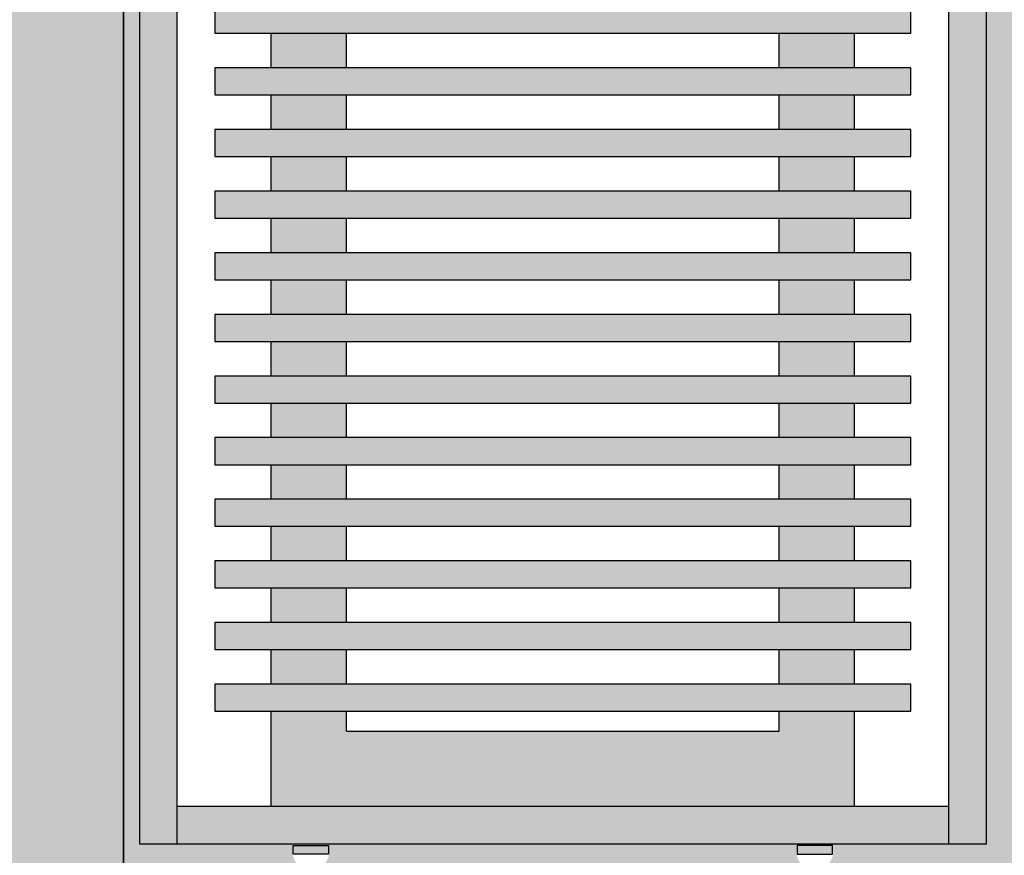
# Model space of a CAD drawing. Units: inches. Extents: x 1704 to 6393, y -157 to 1172.
# Tile 27 of 122: x 2351 to 2377, y 272 to 295. Entities that reach past the tile are written whole.
import ezdxf

# ---------------------------------------------------------------- set-up
doc = ezdxf.new("R2010")
doc.units = ezdxf.units.IN
doc.header["$MEASUREMENT"] = 0
for name, color, linetype, lineweight in [('A-ANNO-DIMS', 7, 'Continuous', 13), ('A-FURN', 8, 'Continuous', 18), ('A-WALL-PATT', 7, 'Continuous', 13), ('estofado', 7, 'Continuous', 25), ('WALLS', 7, 'Continuous', 35)]:
    doc.layers.add(name, color=color, linetype=linetype, lineweight=lineweight)
doc.layers.add('A-FLOR-PATT', color=7, linetype='Continuous', lineweight=13, true_color=0xf2f2f2)
doc.layers.add('MOBIL', color=7, linetype='Continuous')
doc.styles.get("Standard").update_dxf_attribs({"font": 'arial.ttf'})
doc.dimstyles.get("Standard").update_dxf_attribs({"dimtxt": 6, "dimasz": 2, "dimexe": 0.18, "dimexo": 0.0625, "dimgap": 0.09, "dimtad": 0, "dimtih": 1, "dimtoh": 1, "dimdec": 1, "dimzin": 0, "dimdsep": 46, "dimlunit": 3, "dimtxsty": 'Standard', "dimblk": 'ARCHTICK', "dimcen": 0.09, "dimadec": 0, "dimazin": 0, "dimtfac": 1, "dimtdec": 1, "dimtofl": 0, "dimtmove": 0, "dimatfit": 3, "dimfxl": 1, "dimtolj": 1, "dimtzin": 0, "dimarcsym": 0})

# ---------------------------------------------------------------- blocks, each defined once
blk = doc.blocks.new('Aparador Aido WV')
at = {"layer": 'MOBIL'}
h = blk.add_hatch(color=256, dxfattribs=at)
h.set_gradient(color1=(226, 228, 228), one_color=1, tint=1, name='CYLINDER')
h.paths.add_polyline_path([(0.9, -0.02), (0.9, 0), (-0.9, 0), (-0.9, -0.02)])
h = blk.add_hatch(color=256, dxfattribs=at)
h.set_gradient(color1=(226, 228, 228), one_color=1, tint=1)
h.paths.add_polyline_path([(-0.88, -0.02), (-0.9, -0.02), (-0.9, -0.43), (-0.88, -0.43)])
h = blk.add_hatch(color=256, dxfattribs=at)
h.set_gradient(color1=(106, 79, 62), color2=(55, 41, 32), one_color=1, tint=0.17)
h.paths.add_polyline_path([(-0.8151, -0.04017), (-0.82946, -0.04017), (-0.82946, -0.40983), (-0.8151, -0.40983)])
h = blk.add_hatch(color=256, dxfattribs=at)
h.set_gradient(color1=(106, 79, 62), color2=(55, 41, 32), one_color=1, tint=0.17)
h.paths.add_polyline_path([(-0.79671, -0.04017), (-0.79671, -0.40983), (-0.78235, -0.40983), (-0.78235, -0.04017)])
h = blk.add_hatch(color=256, dxfattribs=at)
h.set_gradient(color1=(106, 79, 62), color2=(55, 41, 32), one_color=1, tint=0.17)
h.paths.add_polyline_path([(-0.76396, -0.04017), (-0.76396, -0.40983), (-0.7496, -0.40983), (-0.7496, -0.04017)])
h = blk.add_hatch(color=256, dxfattribs=at)
h.set_gradient(color1=(106, 79, 62), color2=(55, 41, 32), one_color=1, tint=0.17)
h.paths.add_polyline_path([(-0.73121, -0.04017), (-0.73121, -0.40983), (-0.71684, -0.40983), (-0.71684, -0.04017)])
h = blk.add_hatch(color=256, dxfattribs=at)
h.set_gradient(color1=(106, 79, 62), color2=(55, 41, 32), one_color=1, tint=0.17)
h.paths.add_polyline_path([(-0.69846, -0.04017), (-0.69846, -0.40983), (-0.68409, -0.40983), (-0.68409, -0.04017)])
h = blk.add_hatch(color=256, dxfattribs=at)
h.set_gradient(color1=(106, 79, 62), color2=(55, 41, 32), one_color=1, tint=0.17)
h.paths.add_polyline_path([(-0.66571, -0.04017), (-0.66571, -0.40983), (-0.65134, -0.40983), (-0.65134, -0.04017)])
h = blk.add_hatch(color=256, dxfattribs=at)
h.set_gradient(color1=(106, 79, 62), color2=(55, 41, 32), one_color=1, tint=0.17)
h.paths.add_polyline_path([(-0.63295, -0.04017), (-0.63295, -0.40983), (-0.61859, -0.40983), (-0.61859, -0.04017)])
h = blk.add_hatch(color=256, dxfattribs=at)
h.set_gradient(color1=(106, 79, 62), color2=(55, 41, 32), one_color=1, tint=0.17)
h.paths.add_polyline_path([(-0.6002, -0.04017), (-0.6002, -0.40983), (-0.58584, -0.40983), (-0.58584, -0.04017)])
h = blk.add_hatch(color=256, dxfattribs=at)
h.set_gradient(color1=(106, 79, 62), color2=(55, 41, 32), one_color=1, tint=0.17)
h.paths.add_polyline_path([(-0.56745, -0.40983), (-0.55309, -0.40983), (-0.55309, -0.04017), (-0.56745, -0.04017)])
h = blk.add_hatch(color=256, dxfattribs=at)
h.set_gradient(color1=(106, 79, 62), color2=(55, 41, 32), one_color=1, tint=0.17)
h.paths.add_polyline_path([(-0.5347, -0.04017), (-0.5347, -0.40983), (-0.52033, -0.40983), (-0.52033, -0.04017)])
h = blk.add_hatch(color=256, dxfattribs=at)
h.set_gradient(color1=(106, 79, 62), color2=(55, 41, 32), one_color=1, tint=0.17)
h.paths.add_polyline_path([(-0.50195, -0.04017), (-0.50195, -0.40983), (-0.48758, -0.40983), (-0.48758, -0.04017)])
h = blk.add_hatch(color=256, dxfattribs=at)
h.set_gradient(color1=(106, 79, 62), color2=(55, 41, 32), one_color=1, tint=0.17)
h.paths.add_polyline_path([(-0.4692, -0.04017), (-0.4692, -0.40983), (-0.45483, -0.40983), (-0.45483, -0.04017)])
h = blk.add_hatch(color=256, dxfattribs=at)
h.set_gradient(color1=(106, 79, 62), color2=(157, 117, 92), one_color=1, tint=0.49)
h.paths.add_polyline_path([(-0.84, -0.11), (-0.82946, -0.11), (-0.82946, -0.07), (-0.88, -0.07), (-0.88, -0.38), (-0.82946, -0.38), (-0.82946, -0.34), (-0.84, -0.34)])
h = blk.add_hatch(color=256, dxfattribs=at)
h.set_gradient(color1=(106, 79, 62), color2=(157, 117, 92), one_color=1, tint=0.49)
h.paths.add_polyline_path([(-0.79671, -0.07), (-0.8151, -0.07), (-0.8151, -0.11), (-0.79671, -0.11)])
h = blk.add_hatch(color=256, dxfattribs=at)
h.set_gradient(color1=(106, 79, 62), color2=(157, 117, 92), one_color=1, tint=0.49)
h.paths.add_polyline_path([(-0.76396, -0.07), (-0.78235, -0.07), (-0.78235, -0.11), (-0.76396, -0.11)])
h = blk.add_hatch(color=256, dxfattribs=at)
h.set_gradient(color1=(106, 79, 62), color2=(157, 117, 92), one_color=1, tint=0.49)
h.paths.add_polyline_path([(-0.73121, -0.07), (-0.7496, -0.07), (-0.7496, -0.11), (-0.73121, -0.11)])
h = blk.add_hatch(color=256, dxfattribs=at)
h.set_gradient(color1=(106, 79, 62), color2=(157, 117, 92), one_color=1, tint=0.49)
h.paths.add_polyline_path([(-0.69846, -0.07), (-0.71684, -0.07), (-0.71684, -0.11), (-0.69846, -0.11)])
h = blk.add_hatch(color=256, dxfattribs=at)
h.set_gradient(color1=(106, 79, 62), color2=(157, 117, 92), one_color=1, tint=0.49)
h.paths.add_polyline_path([(-0.66571, -0.07), (-0.68409, -0.07), (-0.68409, -0.11), (-0.66571, -0.11)])
h = blk.add_hatch(color=256, dxfattribs=at)
h.set_gradient(color1=(106, 79, 62), color2=(157, 117, 92), one_color=1, tint=0.49)
h.paths.add_polyline_path([(-0.63295, -0.07), (-0.65134, -0.07), (-0.65134, -0.11), (-0.63295, -0.11)])
h = blk.add_hatch(color=256, dxfattribs=at)
h.set_gradient(color1=(106, 79, 62), color2=(157, 117, 92), one_color=1, tint=0.49)
h.paths.add_polyline_path([(-0.6002, -0.07), (-0.61859, -0.07), (-0.61859, -0.11), (-0.6002, -0.11)])
h = blk.add_hatch(color=256, dxfattribs=at)
h.set_gradient(color1=(106, 79, 62), color2=(157, 117, 92), one_color=1, tint=0.49)
h.paths.add_polyline_path([(-0.56745, -0.07), (-0.58584, -0.07), (-0.58584, -0.11), (-0.56745, -0.11)])
h = blk.add_hatch(color=256, dxfattribs=at)
h.set_gradient(color1=(106, 79, 62), color2=(157, 117, 92), one_color=1, tint=0.49)
h.paths.add_polyline_path([(-0.5347, -0.07), (-0.55309, -0.07), (-0.55309, -0.11), (-0.5347, -0.11)])
h = blk.add_hatch(color=256, dxfattribs=at)
h.set_gradient(color1=(106, 79, 62), color2=(157, 117, 92), one_color=1, tint=0.49)
h.paths.add_polyline_path([(-0.50195, -0.07), (-0.52033, -0.07), (-0.52033, -0.11), (-0.50195, -0.11)])
h = blk.add_hatch(color=256, dxfattribs=at)
h.set_gradient(color1=(106, 79, 62), color2=(157, 117, 92), one_color=1, tint=0.49)
h.paths.add_polyline_path([(-0.4692, -0.07), (-0.48758, -0.07), (-0.48758, -0.11), (-0.4692, -0.11)])
h = blk.add_hatch(color=256, dxfattribs=at)
h.set_gradient(color1=(106, 79, 62), color2=(157, 117, 92), one_color=1, tint=0.49)
h.paths.add_polyline_path([(-0.79671, -0.34), (-0.8151, -0.34), (-0.8151, -0.38), (-0.79671, -0.38)])
h = blk.add_hatch(color=256, dxfattribs=at)
h.set_gradient(color1=(106, 79, 62), color2=(157, 117, 92), one_color=1, tint=0.49)
h.paths.add_polyline_path([(-0.76396, -0.34), (-0.78235, -0.34), (-0.78235, -0.38), (-0.76396, -0.38)])
h = blk.add_hatch(color=256, dxfattribs=at)
h.set_gradient(color1=(106, 79, 62), color2=(157, 117, 92), one_color=1, tint=0.49)
h.paths.add_polyline_path([(-0.73121, -0.34), (-0.7496, -0.34), (-0.7496, -0.38), (-0.73121, -0.38)])
h = blk.add_hatch(color=256, dxfattribs=at)
h.set_gradient(color1=(106, 79, 62), color2=(157, 117, 92), one_color=1, tint=0.49)
h.paths.add_polyline_path([(-0.69846, -0.34), (-0.71684, -0.34), (-0.71684, -0.38), (-0.69846, -0.38)])
h = blk.add_hatch(color=256, dxfattribs=at)
h.set_gradient(color1=(106, 79, 62), color2=(157, 117, 92), one_color=1, tint=0.49)
h.paths.add_polyline_path([(-0.66571, -0.34), (-0.68409, -0.34), (-0.68409, -0.38), (-0.66571, -0.38)])
h = blk.add_hatch(color=256, dxfattribs=at)
h.set_gradient(color1=(106, 79, 62), color2=(157, 117, 92), one_color=1, tint=0.49)
h.paths.add_polyline_path([(-0.63295, -0.34), (-0.65134, -0.34), (-0.65134, -0.38), (-0.63295, -0.38)])
h = blk.add_hatch(color=256, dxfattribs=at)
h.set_gradient(color1=(106, 79, 62), color2=(157, 117, 92), one_color=1, tint=0.49)
h.paths.add_polyline_path([(-0.6002, -0.34), (-0.61859, -0.34), (-0.61859, -0.38), (-0.6002, -0.38)])
h = blk.add_hatch(color=256, dxfattribs=at)
h.set_gradient(color1=(106, 79, 62), color2=(157, 117, 92), one_color=1, tint=0.49)
h.paths.add_polyline_path([(-0.56745, -0.34), (-0.58584, -0.34), (-0.58584, -0.38), (-0.56745, -0.38)])
h = blk.add_hatch(color=256, dxfattribs=at)
h.set_gradient(color1=(106, 79, 62), color2=(157, 117, 92), one_color=1, tint=0.49)
h.paths.add_polyline_path([(-0.5347, -0.34), (-0.55309, -0.34), (-0.55309, -0.38), (-0.5347, -0.38)])
h = blk.add_hatch(color=256, dxfattribs=at)
h.set_gradient(color1=(106, 79, 62), color2=(157, 117, 92), one_color=1, tint=0.49)
h.paths.add_polyline_path([(-0.50195, -0.34), (-0.52033, -0.34), (-0.52033, -0.38), (-0.50195, -0.38)])
h = blk.add_hatch(color=256, dxfattribs=at)
h.set_gradient(color1=(106, 79, 62), color2=(157, 117, 92), one_color=1, tint=0.49)
h.paths.add_polyline_path([(-0.4692, -0.34), (-0.48758, -0.34), (-0.48758, -0.38), (-0.4692, -0.38)])
h = blk.add_hatch(color=256, dxfattribs=at)
h.set_gradient(color1=(226, 228, 228), one_color=1, tint=1, name='CYLINDER')
h.paths.add_polyline_path([(0.9, -0.45), (0.9, -0.43), (-0.9, -0.43), (-0.9, -0.45)])
at = {"layer": 'estofado', "ltscale": 0.5}
for p, q in [((-0.88, -0.07), (-0.82946, -0.07)), ((-0.8151, -0.07), (-0.79671, -0.07)), ((-0.78235, -0.07), (-0.76396, -0.07)), ((-0.7496, -0.07), (-0.73121, -0.07)), ((-0.71684, -0.07), (-0.69846, -0.07)), ((-0.68409, -0.07), (-0.66571, -0.07)), ((-0.65134, -0.07), (-0.63295, -0.07)), ((-0.61859, -0.07), (-0.6002, -0.07)), ((-0.58584, -0.07), (-0.56745, -0.07)), ((-0.55309, -0.07), (-0.5347, -0.07)), ((-0.52033, -0.07), (-0.50195, -0.07)), ((-0.48758, -0.07), (-0.4692, -0.07)), ((-0.84, -0.11), (-0.84, -0.34)), ((-0.84, -0.11), (-0.82946, -0.11)), ((-0.8151, -0.11), (-0.79671, -0.11)), ((-0.78235, -0.11), (-0.76396, -0.11)), ((-0.7496, -0.11), (-0.73121, -0.11)), ((-0.71684, -0.11), (-0.69846, -0.11)), ((-0.68409, -0.11), (-0.66571, -0.11)), ((-0.65134, -0.11), (-0.63295, -0.11)), ((-0.61859, -0.11), (-0.6002, -0.11)), ((-0.58584, -0.11), (-0.56745, -0.11)), ((-0.55309, -0.11), (-0.5347, -0.11)), ((-0.52033, -0.11), (-0.50195, -0.11)), ((-0.48758, -0.11), (-0.4692, -0.11)), ((-0.84, -0.34), (-0.82946, -0.34)), ((-0.8151, -0.34), (-0.79671, -0.34)), ((-0.78235, -0.34), (-0.76396, -0.34)), ((-0.7496, -0.34), (-0.73121, -0.34)), ((-0.71684, -0.34), (-0.69846, -0.34)), ((-0.68409, -0.34), (-0.66571, -0.34)), ((-0.65134, -0.34), (-0.63295, -0.34)), ((-0.61859, -0.34), (-0.6002, -0.34)), ((-0.58584, -0.34), (-0.56745, -0.34)), ((-0.55309, -0.34), (-0.5347, -0.34)), ((-0.52033, -0.34), (-0.50195, -0.34)), ((-0.48758, -0.34), (-0.4692, -0.34)), ((-0.88, -0.38), (-0.82946, -0.38)), ((-0.84, -0.38), (-0.82946, -0.38)), ((-0.8151, -0.38), (-0.79671, -0.38)), ((-0.78235, -0.38), (-0.76396, -0.38)), ((-0.7496, -0.38), (-0.73121, -0.38)), ((-0.71684, -0.38), (-0.69846, -0.38)), ((-0.68409, -0.38), (-0.66571, -0.38)), ((-0.65134, -0.38), (-0.63295, -0.38)), ((-0.61859, -0.38), (-0.6002, -0.38)), ((-0.58584, -0.38), (-0.56745, -0.38)), ((-0.55309, -0.38), (-0.5347, -0.38)), ((-0.52033, -0.38), (-0.50195, -0.38)), ((-0.48758, -0.38), (-0.4692, -0.38))]:
    blk.add_line(p, q, dxfattribs=at)
for points in [[(-0.82946, -0.04017), (-0.82946, -0.40983), (-0.8151, -0.40983), (-0.8151, -0.04017)], [(-0.79671, -0.04017), (-0.79671, -0.40983), (-0.78235, -0.40983), (-0.78235, -0.04017)], [(-0.76396, -0.04017), (-0.76396, -0.40983), (-0.7496, -0.40983), (-0.7496, -0.04017)], [(-0.73121, -0.04017), (-0.73121, -0.40983), (-0.71684, -0.40983), (-0.71684, -0.04017)], [(-0.69846, -0.04017), (-0.69846, -0.40983), (-0.68409, -0.40983), (-0.68409, -0.04017)], [(-0.66571, -0.04017), (-0.66571, -0.40983), (-0.65134, -0.40983), (-0.65134, -0.04017)], [(-0.63295, -0.04017), (-0.63295, -0.40983), (-0.61859, -0.40983), (-0.61859, -0.04017)], [(-0.6002, -0.04017), (-0.6002, -0.40983), (-0.58584, -0.40983), (-0.58584, -0.04017)], [(-0.56745, -0.04017), (-0.56745, -0.40983), (-0.55309, -0.40983), (-0.55309, -0.04017)], [(-0.5347, -0.04017), (-0.5347, -0.40983), (-0.52033, -0.40983), (-0.52033, -0.04017)], [(-0.50195, -0.04017), (-0.50195, -0.40983), (-0.48758, -0.40983), (-0.48758, -0.04017)], [(-0.4692, -0.04017), (-0.4692, -0.40983), (-0.45483, -0.40983), (-0.45483, -0.04017)], [(-0.90536, -0.0817), (-0.90086, -0.0817), (-0.90086, -0.10055), (-0.90536, -0.10055)], [(-0.90536, -0.3683), (-0.90086, -0.3683), (-0.90086, -0.34945), (-0.90536, -0.34945)]]:
    blk.add_lwpolyline(points, close=True, dxfattribs=at)
at = {"layer": 'MOBIL'}
for p, q in [((0.9, -0.02), (-0.9, -0.02)), ((-0.88, -0.02), (-0.88, -0.43)), ((-0.9, -0.43), (0.9, -0.43))]:
    blk.add_line(p, q, dxfattribs=at)
blk.add_lwpolyline([(-0.9, -0.45), (0.9, -0.45), (0.9, 0), (-0.9, 0)], close=True, dxfattribs=at)
blk = doc.blocks.new('_ArchTick')
at = {"color": 0, "linetype": 'ByBlock', "const_width": 0.15}
blk.add_lwpolyline([(-0.5, -0.5), (0.5, 0.5)], dxfattribs=at)
blk = doc.blocks.new('*D68')
at = {"layer": 'A-ANNO-DIMS', "color": 0, "lineweight": -2, "transparency": 16777216}
for p, q in [((2353.706, 363.767), (2339.834, 363.767)), ((2340.014, 363.767), (2340.014, 321.111)), ((2340.014, 272.066), (2340.014, 314.722)), ((2353.706, 272.066), (2339.834, 272.066))]:
    blk.add_line(p, q, dxfattribs=at)
at = {"layer": 'Defpoints', "color": 0, "lineweight": -3, "transparency": 16777216}
for p in [(2340.014, 363.767), (2353.769, 363.767), (2353.769, 272.066)]:
    blk.add_point(p, dxfattribs=at)
at = {"layer": 'A-ANNO-DIMS', "color": 0, "lineweight": -2, "transparency": 16777216, "xscale": 2, "yscale": 2, "zscale": 2}
for p, rotation in [((2340.014, 363.767), 90), ((2340.014, 272.066), 270)]:
    blk.add_blockref('_ArchTick', p, dxfattribs=dict(at, rotation=rotation))
at = {"layer": 'A-ANNO-DIMS', "color": 0, "transparency": 16777216, "insert": (2340.014, 317.916), "char_height": 6, "attachment_point": 5}
blk.add_mtext('\\A1;SIDEBOARD 92', dxfattribs=at)
blk = doc.blocks.new('*D93')
at = {"layer": 'A-ANNO-DIMS', "color": 0, "lineweight": -2, "transparency": 16777216}
for p, q in [((2605.286, 895.213), (1829.698, 895.213)), ((1829.878, 895.213), (1829.878, 495.866)), ((1829.878, 90.213), (1829.878, 489.56)), ((2605.286, 90.213), (1829.698, 90.213))]:
    blk.add_line(p, q, dxfattribs=at)
at = {"layer": 'Defpoints', "color": 0, "lineweight": -3, "transparency": 16777216}
for p in [(2605.349, 895.213), (1829.878, 90.213), (2605.349, 90.213)]:
    blk.add_point(p, dxfattribs=at)
at = {"layer": 'A-ANNO-DIMS', "color": 0, "lineweight": -2, "transparency": 16777216, "xscale": 2, "yscale": 2, "zscale": 2}
for p, rotation in [((1829.878, 895.213), 90), ((1829.878, 90.213), 270)]:
    blk.add_blockref('_ArchTick', p, dxfattribs=dict(at, rotation=rotation))
at = {"layer": 'A-ANNO-DIMS', "color": 0, "transparency": 16777216, "insert": (1829.878, 492.713), "char_height": 6, "attachment_point": 5}
blk.add_mtext('\\A1;805', dxfattribs=at)

msp = doc.modelspace()

# ---------------------------------------------------------------- hatches: boundary and pattern name
at = {"layer": 'A-FLOR-PATT', "transparency": 33554528}
h = msp.add_hatch(color=256, dxfattribs=at)
h.dxf.hatch_style = 1
h.paths.add_polyline_path([(2325.349, 863.213), (2325.349, 887.213), (2263.349, 887.213), (2167.349, 887.213), (2081.349, 887.213), (2081.349, 719.213), (2277.349, 719.213), (2277.349, 711.213), (2277.349, 372.213), (2349.349, 372.213), (2381.349, 372.213), (2381.349, 364.213), (2353.349, 364.213), (2353.349, 270.213), (2381.349, 270.213), (2381.349, 266.213), (2357.349, 266.213), (2357.349, 98.213), (2381.349, 98.213), (2385.181, 98.213), (2386.482, 98.213), (2424.215, 98.213), (2425.516, 98.213), (2429.349, 98.213), (2597.349, 98.213), (2597.349, 146.213), (2597.349, 218.213), (2597.349, 266.213), (2423.349, 266.213), (2423.349, 270.213), (2473.349, 270.213), (2473.349, 294.213), (2477.349, 294.213), (2477.349, 270.213), (2547.349, 270.213), (2547.349, 364.213), (2477.349, 364.213), (2477.349, 318.213), (2473.349, 318.213), (2473.349, 364.213), (2423.349, 364.213), (2423.349, 372.213), (2469.349, 372.213), (2469.349, 459.213), (2469.349, 538.213), (2350.349, 538.213), (2350.349, 565.713), (2358.349, 565.713), (2358.349, 545.213), (2420.349, 545.213), (2420.349, 610.213), (2358.349, 610.213), (2358.349, 589.713), (2350.349, 589.713), (2350.349, 615.213), (2425.349, 615.213), (2425.349, 607.213), (2425.349, 546.213), (2469.349, 546.213), (2514.349, 546.213), (2514.349, 607.213), (2449.349, 607.213), (2449.349, 615.213), (2451.738, 615.213), (2451.738, 659.213), (2427.738, 659.213), (2427.738, 665.213), (2367.738, 665.213), (2367.738, 667.213), (2367.738, 711.213), (2325.349, 711.213), (2325.349, 719.213), (2325.349, 755.213), (2325.349, 763.213)])
h.paths.add_polyline_path([(2233.858, 822.533, -0.187247), (2233.858, 809.14), (2231.697, 808.804, 0.084893), (2233.131, 814.486), (2230.424, 814.486, -0.104258), (2228.553, 808.313), (2217.751, 807.156, -0.222222), (2217.751, 824.517), (2228.553, 823.359, -0.104258), (2230.424, 817.186), (2233.131, 817.186, 0.084893), (2231.697, 822.868)], flags=16)
h.paths.add_polyline_path([(2213.621, 833.197), (2213.621, 798.475), (2156.048, 798.475), (2156.048, 833.197)], flags=16)
h.paths.add_polyline_path([(2203.932, 848.099), (2205.089, 837.296, -0.222222), (2187.728, 837.296), (2188.885, 848.099, -0.104258), (2195.058, 849.969), (2195.058, 852.676, 0.084893), (2189.377, 851.242), (2189.712, 853.404, -0.187247), (2203.105, 853.404), (2203.44, 851.242, 0.084893), (2197.759, 852.676), (2197.759, 849.969, -0.104258)], flags=16)
h.paths.add_polyline_path([(2181.941, 837.296, -0.222222), (2164.58, 837.296), (2165.737, 848.099, -0.104258), (2171.91, 849.969), (2171.91, 852.676, 0.084893), (2166.229, 851.242), (2166.564, 853.404, -0.187247), (2179.957, 853.404), (2180.292, 851.242, 0.084893), (2174.611, 852.676), (2174.611, 849.969, -0.104258), (2180.784, 848.099)], flags=16)
h.paths.add_polyline_path([(2205.089, 794.376), (2203.932, 783.574, -0.104258), (2197.759, 781.703), (2197.759, 778.996, 0.084893), (2203.44, 780.43), (2203.105, 778.269, -0.187247), (2189.712, 778.269), (2189.377, 780.43, 0.084893), (2195.058, 778.996), (2195.058, 781.703, -0.104258), (2188.885, 783.574), (2187.728, 794.376, -0.222222)], flags=16)
h.paths.add_polyline_path([(2181.941, 794.376), (2180.784, 783.574, -0.104258), (2174.611, 781.703), (2174.611, 778.996, 0.084893), (2180.292, 780.43), (2179.957, 778.269, -0.187247), (2166.564, 778.269), (2166.229, 780.43, 0.084893), (2171.91, 778.996), (2171.91, 781.703, -0.104258), (2165.737, 783.574), (2164.58, 794.376, -0.222222)], flags=16)
h.paths.add_polyline_path([(2151.918, 807.156), (2141.116, 808.313, -0.104258), (2139.245, 814.486), (2136.539, 814.486, 0.084893), (2137.972, 808.804), (2135.811, 809.14, -0.187247), (2135.811, 822.533), (2137.972, 822.868, 0.084893), (2136.539, 817.186), (2139.245, 817.186, -0.104258), (2141.116, 823.359), (2151.918, 824.517, -0.222222)], flags=16)
h.paths.add_polyline_path([(2357.868, 363.41), (2358.814, 363.41, 0.75376)], flags=16)
h.paths.add_polyline_path([(2372.241, 363.117), (2372.248, 363.117), (2372.248, 363.343), (2371.302, 363.343), (2371.302, 363.139, -1.360391)], flags=16)
h.paths.add_polyline_path([(2371.309, 272.716), (2371.302, 272.716), (2371.302, 272.49), (2372.248, 272.49), (2372.248, 272.693, -1.360391)], flags=16)
h.paths.add_polyline_path([(2357.875, 272.716), (2357.868, 272.716), (2357.868, 272.49), (2358.814, 272.49), (2358.814, 272.693, -1.360391)], flags=16)
h.paths.add_polyline_path([(2353.769, 363.074), (2376.347, 363.074), (2376.347, 272.759), (2353.769, 272.759)], flags=16)
h.paths.add_polyline_path([(2354.772, 362.07), (2375.344, 362.07), (2375.344, 273.762), (2354.772, 273.762)], flags=0)
h.paths.add_polyline_path([(2357.868, 363.343), (2358.814, 363.343), (2358.814, 363.117), (2357.868, 363.117)], flags=16)
h.paths.add_polyline_path([(2359.288, 359.184), (2359.288, 360.063), (2370.828, 360.063), (2370.828, 359.184), (2374.332, 359.184), (2374.332, 358.464), (2372.835, 358.464), (2372.835, 357.541), (2374.332, 357.541), (2374.332, 356.82), (2372.835, 356.82), (2372.835, 355.898), (2374.332, 355.898), (2374.332, 355.177), (2372.835, 355.177), (2372.835, 354.254), (2374.332, 354.254), (2374.332, 353.534), (2372.835, 353.534), (2372.835, 352.611), (2374.332, 352.611), (2374.332, 351.89), (2372.835, 351.89), (2372.835, 350.968), (2374.332, 350.968), (2374.332, 350.247), (2372.835, 350.247), (2372.835, 349.324), (2374.332, 349.324), (2374.332, 348.604), (2372.835, 348.604), (2372.835, 347.681), (2374.332, 347.681), (2374.332, 346.96), (2372.835, 346.96), (2372.835, 346.038), (2374.332, 346.038), (2374.332, 345.317), (2372.835, 345.317), (2372.835, 344.395), (2374.332, 344.395), (2374.332, 343.674), (2372.835, 343.674), (2372.835, 342.751), (2374.332, 342.751), (2374.332, 342.03), (2372.835, 342.03), (2372.835, 341.108), (2374.332, 341.108), (2374.332, 340.387), (2372.835, 340.387), (2372.835, 339.465), (2374.332, 339.465), (2374.332, 338.744), (2372.835, 338.744), (2372.835, 337.821), (2374.332, 337.821), (2374.332, 337.1), (2372.835, 337.1), (2372.835, 336.178), (2374.332, 336.178), (2374.332, 335.457), (2372.835, 335.457), (2372.835, 334.535), (2374.332, 334.535), (2374.332, 333.814), (2372.835, 333.814), (2372.835, 332.891), (2374.332, 332.891), (2374.332, 332.171), (2372.835, 332.171), (2372.835, 331.248), (2374.332, 331.248), (2374.332, 330.527), (2372.835, 330.527), (2372.835, 329.605), (2374.332, 329.605), (2374.332, 328.884), (2372.835, 328.884), (2372.835, 327.961), (2374.332, 327.961), (2374.332, 327.241), (2372.835, 327.241), (2372.835, 326.318), (2374.332, 326.318), (2374.332, 325.597), (2372.835, 325.597), (2372.835, 324.675), (2374.332, 324.675), (2374.332, 323.954), (2372.835, 323.954), (2372.835, 323.031), (2374.332, 323.031), (2374.332, 322.311), (2372.835, 322.311), (2372.835, 321.388), (2374.332, 321.388), (2374.332, 320.667), (2372.835, 320.667), (2372.835, 319.745), (2374.332, 319.745), (2374.332, 319.024), (2372.835, 319.024), (2372.835, 318.102), (2374.332, 318.102), (2374.332, 317.381), (2372.835, 317.381), (2372.835, 316.458), (2374.332, 316.458), (2374.332, 315.737), (2372.835, 315.737), (2372.835, 314.815), (2374.332, 314.815), (2374.332, 314.094), (2372.835, 314.094), (2372.835, 313.172), (2374.332, 313.172), (2374.332, 312.451), (2372.835, 312.451), (2372.835, 311.528), (2374.332, 311.528), (2374.332, 310.807), (2372.835, 310.807), (2372.835, 309.885), (2374.332, 309.885), (2374.332, 309.164), (2372.835, 309.164), (2372.835, 308.242), (2374.332, 308.242), (2374.332, 307.521), (2372.835, 307.521), (2372.835, 306.598), (2374.332, 306.598), (2374.332, 305.878), (2372.835, 305.878), (2372.835, 304.955), (2374.332, 304.955), (2374.332, 304.234), (2372.835, 304.234), (2372.835, 303.312), (2374.332, 303.312), (2374.332, 302.591), (2372.835, 302.591), (2372.835, 301.668), (2374.332, 301.668), (2374.332, 300.948), (2372.835, 300.948), (2372.835, 300.025), (2374.332, 300.025), (2374.332, 299.304), (2372.835, 299.304), (2372.835, 298.382), (2374.332, 298.382), (2374.332, 297.661), (2372.835, 297.661), (2372.835, 296.738), (2374.332, 296.738), (2374.332, 296.018), (2372.835, 296.018), (2372.835, 295.095), (2374.332, 295.095), (2374.332, 294.374), (2372.835, 294.374), (2372.835, 293.452), (2374.332, 293.452), (2374.332, 292.731), (2372.835, 292.731), (2372.835, 291.809), (2374.332, 291.809), (2374.332, 291.088), (2372.835, 291.088), (2372.835, 290.165), (2374.332, 290.165), (2374.332, 289.444), (2372.835, 289.444), (2372.835, 288.522), (2374.332, 288.522), (2374.332, 287.801), (2372.835, 287.801), (2372.835, 286.879), (2374.332, 286.879), (2374.332, 286.158), (2372.835, 286.158), (2372.835, 285.235), (2374.332, 285.235), (2374.332, 284.514), (2372.835, 284.514), (2372.835, 283.592), (2374.332, 283.592), (2374.332, 282.871), (2372.835, 282.871), (2372.835, 281.949), (2374.332, 281.949), (2374.332, 281.228), (2372.835, 281.228), (2372.835, 280.305), (2374.332, 280.305), (2374.332, 279.585), (2372.835, 279.585), (2372.835, 278.662), (2374.332, 278.662), (2374.332, 277.941), (2372.835, 277.941), (2372.835, 277.019), (2374.332, 277.019), (2374.332, 276.298), (2370.828, 276.298), (2370.828, 275.769), (2359.288, 275.769), (2359.288, 276.298), (2355.784, 276.298), (2355.784, 277.019), (2357.281, 277.019), (2357.281, 277.941), (2355.784, 277.941), (2355.784, 278.662), (2357.281, 278.662), (2357.281, 279.585), (2355.784, 279.585), (2355.784, 280.305), (2357.281, 280.305), (2357.281, 281.228), (2355.784, 281.228), (2355.784, 281.949), (2357.281, 281.949), (2357.281, 282.871), (2355.784, 282.871), (2355.784, 283.592), (2357.281, 283.592), (2357.281, 284.514), (2355.784, 284.514), (2355.784, 285.235), (2357.281, 285.235), (2357.281, 286.158), (2355.784, 286.158), (2355.784, 286.879), (2357.281, 286.879), (2357.281, 287.801), (2355.784, 287.801), (2355.784, 288.522), (2357.281, 288.522), (2357.281, 289.444), (2355.784, 289.444), (2355.784, 290.165), (2357.281, 290.165), (2357.281, 291.088), (2355.784, 291.088), (2355.784, 291.809), (2357.281, 291.809), (2357.281, 292.731), (2355.784, 292.731), (2355.784, 293.452), (2357.281, 293.452), (2357.281, 294.374), (2355.784, 294.374), (2355.784, 295.095), (2357.281, 295.095), (2357.281, 296.018), (2355.784, 296.018), (2355.784, 296.738), (2357.281, 296.738), (2357.281, 297.661), (2355.784, 297.661), (2355.784, 298.382), (2357.281, 298.382), (2357.281, 299.304), (2355.784, 299.304), (2355.784, 300.025), (2357.281, 300.025), (2357.281, 300.948), (2355.784, 300.948), (2355.784, 301.668), (2357.281, 301.668), (2357.281, 302.591), (2355.784, 302.591), (2355.784, 303.312), (2357.281, 303.312), (2357.281, 304.234), (2355.784, 304.234), (2355.784, 304.955), (2357.281, 304.955), (2357.281, 305.878), (2355.784, 305.878), (2355.784, 306.598), (2357.281, 306.598), (2357.281, 307.521), (2355.784, 307.521), (2355.784, 308.242), (2357.281, 308.242), (2357.281, 309.164), (2355.784, 309.164), (2355.784, 309.885), (2357.281, 309.885), (2357.281, 310.807), (2355.784, 310.807), (2355.784, 311.528), (2357.281, 311.528), (2357.281, 312.451), (2355.784, 312.451), (2355.784, 313.172), (2357.281, 313.172), (2357.281, 314.094), (2355.784, 314.094), (2355.784, 314.815), (2357.281, 314.815), (2357.281, 315.737), (2355.784, 315.737), (2355.784, 316.458), (2357.281, 316.458), (2357.281, 317.381), (2355.784, 317.381), (2355.784, 318.102), (2357.281, 318.102), (2357.281, 319.024), (2355.784, 319.024), (2355.784, 319.745), (2357.281, 319.745), (2357.281, 320.667), (2355.784, 320.667), (2355.784, 321.388), (2357.281, 321.388), (2357.281, 322.311), (2355.784, 322.311), (2355.784, 323.031), (2357.281, 323.031), (2357.281, 323.954), (2355.784, 323.954), (2355.784, 324.675), (2357.281, 324.675), (2357.281, 325.597), (2355.784, 325.597), (2355.784, 326.318), (2357.281, 326.318), (2357.281, 327.241), (2355.784, 327.241), (2355.784, 327.961), (2357.281, 327.961), (2357.281, 328.884), (2355.784, 328.884), (2355.784, 329.605), (2357.281, 329.605), (2357.281, 330.527), (2355.784, 330.527), (2355.784, 331.248), (2357.281, 331.248), (2357.281, 332.171), (2355.784, 332.171), (2355.784, 332.891), (2357.281, 332.891), (2357.281, 333.814), (2355.784, 333.814), (2355.784, 334.535), (2357.281, 334.535), (2357.281, 335.457), (2355.784, 335.457), (2355.784, 336.178), (2357.281, 336.178), (2357.281, 337.1), (2355.784, 337.1), (2355.784, 337.821), (2357.281, 337.821), (2357.281, 338.744), (2355.784, 338.744), (2355.784, 339.465), (2357.281, 339.465), (2357.281, 340.387), (2355.784, 340.387), (2355.784, 341.108), (2357.281, 341.108), (2357.281, 342.03), (2355.784, 342.03), (2355.784, 342.751), (2357.281, 342.751), (2357.281, 343.674), (2355.784, 343.674), (2355.784, 344.395), (2357.281, 344.395), (2357.281, 345.317), (2355.784, 345.317), (2355.784, 346.038), (2357.281, 346.038), (2357.281, 346.96), (2355.784, 346.96), (2355.784, 347.681), (2357.281, 347.681), (2357.281, 348.604), (2355.784, 348.604), (2355.784, 349.324), (2357.281, 349.324), (2357.281, 350.247), (2355.784, 350.247), (2355.784, 350.968), (2357.281, 350.968), (2357.281, 351.89), (2355.784, 351.89), (2355.784, 352.611), (2357.281, 352.611), (2357.281, 353.534), (2355.784, 353.534), (2355.784, 354.254), (2357.281, 354.254), (2357.281, 355.177), (2355.784, 355.177), (2355.784, 355.898), (2357.281, 355.898), (2357.281, 356.82), (2355.784, 356.82), (2355.784, 357.541), (2357.281, 357.541), (2357.281, 358.464), (2355.784, 358.464), (2355.784, 359.184)], flags=0)
at = {"layer": 'A-WALL-PATT', "transparency": 33554643}
h = msp.add_hatch(color=256, dxfattribs=at)
h.dxf.hatch_style = 1
h.paths.add_polyline_path([(2167.349, 895.213), (2073.349, 895.213), (2073.349, 887.213), (2081.349, 887.213), (2167.349, 887.213)])
h.paths.add_polyline_path([(2465.349, 895.213), (2273.349, 895.213), (2273.349, 903.213), (2263.349, 903.213), (2263.349, 895.213), (2263.349, 887.213), (2325.349, 887.213), (2325.349, 863.213), (2333.349, 863.213), (2333.349, 887.213), (2465.349, 887.213)])
h.paths.add_polyline_path([(2533.349, 895.213), (2513.349, 895.213), (2513.349, 887.213), (2513.349, 861.213), (2517.349, 861.213), (2517.349, 887.213), (2533.349, 887.213)])
h.paths.add_polyline_path([(2605.349, 895.213), (2581.349, 895.213), (2581.349, 887.213), (2597.349, 887.213), (2597.349, 854.213), (2605.349, 854.213)])
h.paths.add_polyline_path([(2605.349, 752.213), (2629.349, 752.213), (2629.349, 716.213), (2605.349, 716.213), (2605.349, 712.213), (2719.349, 712.213), (2719.349, 716.213), (2631.349, 716.213), (2631.349, 754.213), (2605.349, 754.213), (2605.349, 794.213), (2597.349, 794.213), (2597.349, 787.213), (2517.349, 787.213), (2517.349, 813.213), (2513.349, 813.213), (2513.349, 783.213), (2517.349, 783.213), (2597.349, 783.213), (2597.349, 719.213), (2517.349, 719.213), (2517.349, 753.213), (2513.349, 753.213), (2513.349, 719.213), (2365.349, 719.213), (2365.349, 763.213), (2325.349, 763.213), (2325.349, 755.213), (2357.349, 755.213), (2357.349, 719.213), (2325.349, 719.213), (2325.349, 711.213), (2547.349, 711.213), (2547.349, 615.213), (2449.349, 615.213), (2449.349, 607.213), (2514.349, 607.213), (2514.349, 546.213), (2439.349, 546.213), (2425.349, 546.213), (2425.349, 607.213), (2425.349, 615.213), (2350.349, 615.213), (2350.349, 589.713), (2358.349, 589.713), (2358.349, 610.213), (2420.349, 610.213), (2420.349, 545.213), (2358.349, 545.213), (2358.349, 565.713), (2350.349, 565.713), (2350.349, 538.213), (2469.349, 538.213), (2469.349, 459.213), (2469.349, 372.213), (2423.349, 372.213), (2423.349, 364.213), (2473.349, 364.213), (2473.349, 318.213), (2477.349, 318.213), (2477.349, 364.213), (2547.349, 364.213), (2547.349, 352.213), (2549.349, 352.213), (2549.349, 364.213), (2597.349, 364.213), (2597.349, 328.213), (2549.349, 328.213), (2547.349, 328.213), (2547.349, 326.213), (2549.349, 326.213), (2597.349, 326.213), (2605.349, 326.213), (2605.349, 377.057), (2597.349, 377.057), (2597.349, 372.213), (2477.349, 372.213), (2477.349, 451.213), (2597.349, 451.213), (2605.349, 451.213), (2605.349, 459.213), (2597.349, 459.213), (2477.349, 459.213), (2477.349, 538.213), (2597.349, 538.213), (2597.349, 495.213), (2605.349, 495.213), (2605.349, 512.213), (2631.349, 512.213), (2631.349, 568.213), (2605.349, 568.213), (2605.349, 577.213), (2597.349, 577.213), (2597.349, 542.213), (2518.349, 542.213), (2518.349, 607.213), (2532.349, 607.213), (2605.349, 607.213), (2605.349, 615.213), (2597.349, 615.213), (2551.349, 615.213), (2551.349, 711.213), (2597.349, 711.213), (2597.349, 645.213), (2605.349, 645.213), (2605.349, 712.213), (2605.349, 716.213)])
h.paths.add_polyline_path([(2605.349, 566.213), (2629.349, 566.213), (2629.349, 514.213), (2605.349, 514.213)], flags=16)
h.paths.add_polyline_path([(2381.349, 372.213), (2349.349, 372.213), (2349.349, 202.213), (2337.349, 202.213), (2337.349, 194.213), (2349.349, 194.213), (2349.349, 90.213), (2349.349, 72.213), (2357.349, 72.213), (2357.349, 90.213), (2381.349, 90.213), (2381.349, 98.213), (2357.349, 98.213), (2357.349, 266.213), (2381.349, 266.213), (2381.349, 270.213), (2353.349, 270.213), (2353.349, 364.213), (2381.349, 364.213)])
h.paths.add_polyline_path([(2605.349, 302.213), (2597.349, 302.213), (2597.349, 270.213), (2477.349, 270.213), (2477.349, 294.213), (2473.349, 294.213), (2473.349, 270.213), (2423.349, 270.213), (2423.349, 266.213), (2597.349, 266.213), (2597.349, 218.213), (2605.349, 218.213)])
h.paths.add_polyline_path([(2605.349, 146.213), (2597.349, 146.213), (2597.349, 98.213), (2429.349, 98.213), (2429.349, 90.213), (2597.349, 90.213), (2597.349, 72.213), (2605.349, 72.213), (2605.349, 90.213)])
h.paths.add_polyline_path([(2225.349, 202.213), (2049.349, 202.213), (2049.349, 194.213), (2225.349, 194.213)])
h.paths.add_polyline_path([(2289.349, 202.213), (2277.349, 202.213), (2273.349, 202.213), (2269.516, 202.213), (2269.516, 194.213), (2273.349, 194.213), (2277.349, 194.213), (2289.349, 194.213)])
h.paths.add_polyline_path([(2273.349, 372.213), (2029.19, 372.213), (2029.19, 364.213), (2273.349, 364.213)])
h.paths.add_polyline_path([(2277.349, 545.213), (2213.349, 545.213), (2213.349, 573.213), (2205.349, 573.213), (2177.349, 573.213), (2177.349, 545.213), (2073.349, 545.213), (2073.349, 538.213), (2081.349, 538.213), (2277.349, 538.213)])
h.paths.add_polyline_path([(2181.349, 545.213), (2181.349, 569.213), (2205.349, 569.213), (2205.349, 545.213)], flags=16)
h.paths.add_polyline_path([(2277.349, 719.213), (2081.349, 719.213), (2073.349, 719.213), (2073.349, 711.213), (2154.575, 711.213), (2205.349, 711.213), (2205.349, 687.213), (2205.349, 629.213), (2213.349, 629.213), (2273.349, 629.213), (2273.349, 631.213), (2207.349, 631.213), (2207.349, 707.213), (2231.349, 707.213), (2231.349, 709.213), (2207.349, 709.213), (2207.349, 711.213), (2277.349, 711.213)])

# ---------------------------------------------------------------- linework, layer by layer
at = {"layer": 'WALLS'}
msp.add_line((2353.349, 270.213), (2353.349, 364.213), dxfattribs=at)

# ---------------------------------------------------------------- block references
at = {"layer": 'A-FURN', "xscale": 50.174952135231, "yscale": 50.174952135231, "zscale": 50.174952135231, "rotation": 90}
msp.add_blockref('Aparador Aido WV', (2353.769, 317.916), dxfattribs=at)

# ---------------------------------------------------------------- dimensions: what is measured, and where the dimension line sits
at = {"layer": 'A-ANNO-DIMS'}
dim = msp.add_linear_dim(base=(1829.878, 90.213), p1=(2605.349, 895.213), p2=(2605.349, 90.213), angle=90, dimstyle='Standard', override={"dimdec": 0, "dimlfac": 1, "dimrnd": 0, "dimzin": 0, "dimdsep": 46, "dimlunit": 2}, dxfattribs=at)
dim.commit()
dim.dimension.update_dxf_attribs({"geometry": '*D93', "text_midpoint": (1829.878, 492.713)})
dim = msp.add_linear_dim(base=(2340.014, 363.767), p1=(2353.769, 272.066), p2=(2353.769, 363.767), angle=90, text='SIDEBOARD <>', dimstyle='Standard', override={"dimdec": 0, "dimlfac": 1, "dimrnd": 0, "dimzin": 0, "dimdsep": 46, "dimlunit": 2}, dxfattribs=at)
dim.commit()
dim.dimension.update_dxf_attribs({"geometry": '*D68', "text_midpoint": (2340.014, 317.916)})

doc.saveas('drawing.dxf')
